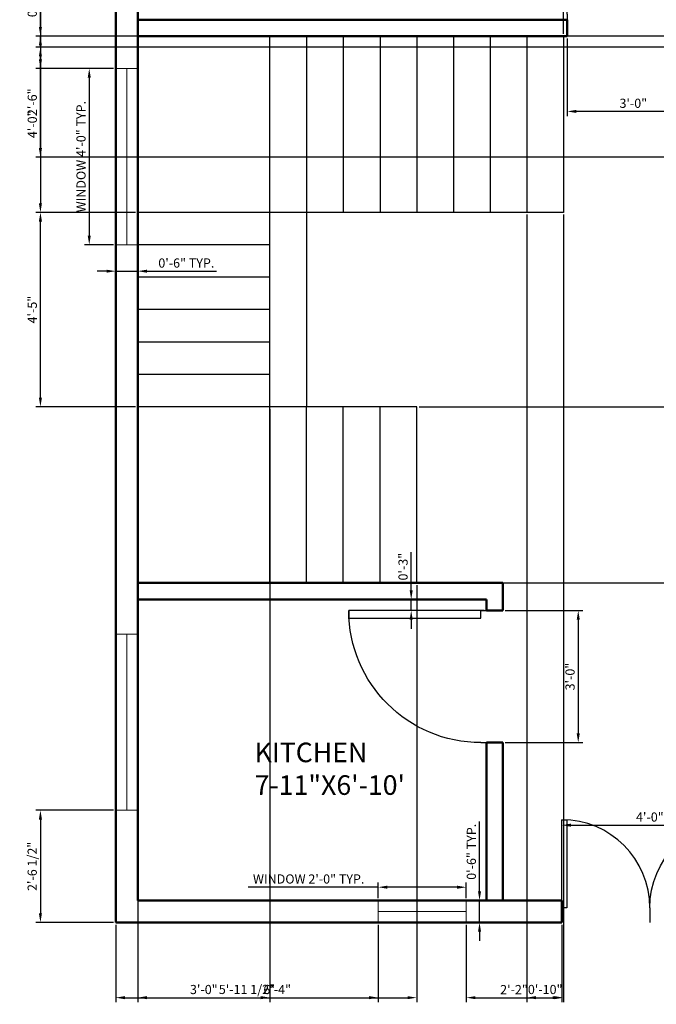
# Model space of a CAD drawing. Units: inches. Extents: x 158445 to 158806, y 254100 to 254533.
# Tile 1 of 3: x 158445 to 158619, y 254100 to 254369. Entities that reach past the tile are written whole.
import ezdxf

# ---------------------------------------------------------------- set-up
doc = ezdxf.new("R2010")
doc.units = ezdxf.units.IN
for name, color, linetype, lineweight in [('A-ANNO-DIMS', 2, 'Continuous', 18), ('A-AREA-IDEN', 7, 'Continuous', 25), ('A-DOOR', 3, 'Continuous', 25), ('A-FLOR-STRS', 7, 'Continuous', 25), ('A-GLAZ', 4, 'Continuous', 18), ('A-WALL', 7, 'Continuous', 50)]:
    doc.layers.add(name, color=color, linetype=linetype, lineweight=lineweight)
doc.styles.get("Standard").update_dxf_attribs({"font": 'arial.ttf'})
doc.dimstyles.new('ISO-25', dxfattribs={"dimtxt": 2.5, "dimasz": 2.5, "dimexe": 1.25, "dimexo": 0.625, "dimtad": 1, "dimlunit": 4, "dimtxsty": 'Standard', "dimcen": 2.5, "dimadec": 0, "dimazin": 0, "dimtfac": 1, "dimtmove": 0, "dimatfit": 3, "dimfxl": 1, "dimarcsym": 0})

# ---------------------------------------------------------------- blocks, each defined once
blk = doc.blocks.new('*U2')
for p, q in [((0, 0), (0, -5)), ((30, 0), (30, -5))]:
    blk.add_line(p, q)
blk.add_lwpolyline([(0, 0), (0, 30), (1.75, 30), (1.75, 0)], close=True)
blk.add_arc((0, 0), 30, 0, 90)
blk = doc.blocks.new('WIN-48IN')
for p, q in [((0, 6), (0, 0)), ((48, 6), (48, 0)), ((0, 3), (48, 3))]:
    blk.add_line(p, q)
blk = doc.blocks.new('WIN-24IN')
for p, q in [((0, 24), (6, 24)), ((3, 0), (3, 24)), ((0, 0), (6, 0))]:
    blk.add_line(p, q)
blk = doc.blocks.new('*D12')
at = {"layer": 'A-ANNO-DIMS', "color": 0, "lineweight": -2, "transparency": 16777216}
for p, q in [((158470.76, 254355.39), (158462.93, 254355.39)), ((158464.18, 254352.89), (158464.18, 254309.89)), ((158470.76, 254307.39), (158462.93, 254307.39))]:
    blk.add_line(p, q, dxfattribs=at)
at = {"layer": 'A-ANNO-DIMS', "color": 0, "transparency": 16777216}
for points in [[(158463.76, 254352.89), (158464.6, 254352.89), (158464.18, 254355.39)], [(158463.76, 254309.89), (158464.6, 254309.89), (158464.18, 254307.39)]]:
    blk.add_solid(points, dxfattribs=at)
at = {"layer": 'Defpoints', "color": 0, "transparency": 16777216}
for p in [(158471.38, 254355.39), (158464.18, 254307.39), (158471.38, 254307.39)]:
    blk.add_point(p, dxfattribs=at)
at = {"layer": 'A-ANNO-DIMS', "color": 0, "transparency": 16777216, "insert": (158462.26, 254331.39), "char_height": 2.5, "attachment_point": 5, "rotation": 90}
blk.add_mtext('WINDOW 4\'-0" TYP.', dxfattribs=at)
blk = doc.blocks.new('*D13')
at = {"layer": 'A-ANNO-DIMS', "color": 0, "lineweight": -2, "transparency": 16777216}
for p, q in [((158471.38, 254306.76), (158471.38, 254298.94)), ((158477.38, 254306.76), (158477.38, 254298.94)), ((158468.88, 254300.19), (158466.38, 254300.19)), ((158471.38, 254300.19), (158477.38, 254300.19)), ((158479.88, 254300.19), (158498.87, 254300.19))]:
    blk.add_line(p, q, dxfattribs=at)
at = {"layer": 'A-ANNO-DIMS', "color": 0, "transparency": 16777216}
for points in [[(158468.88, 254300.6), (158468.88, 254299.77), (158471.38, 254300.19)], [(158479.88, 254300.6), (158479.88, 254299.77), (158477.38, 254300.19)]]:
    blk.add_solid(points, dxfattribs=at)
at = {"layer": 'Defpoints', "color": 0, "transparency": 16777216}
for p in [(158471.38, 254307.39), (158477.38, 254307.39), (158477.38, 254300.19)]:
    blk.add_point(p, dxfattribs=at)
at = {"layer": 'A-ANNO-DIMS', "color": 0, "transparency": 16777216, "insert": (158490.63, 254302.09), "char_height": 2.5, "attachment_point": 5}
blk.add_mtext('0\'-6" TYP.', dxfattribs=at)
blk = doc.blocks.new('*D14')
at = {"layer": 'A-ANNO-DIMS', "color": 0, "lineweight": -2, "transparency": 16777216}
for p, q in [((158542.89, 254129.35), (158542.89, 254133.57)), ((158566.89, 254129.35), (158566.89, 254133.57)), ((158542.89, 254132.32), (158507.5, 254132.32)), ((158564.39, 254132.32), (158545.39, 254132.32))]:
    blk.add_line(p, q, dxfattribs=at)
at = {"layer": 'A-ANNO-DIMS', "color": 0, "transparency": 16777216}
for points in [[(158545.39, 254132.74), (158545.39, 254131.9), (158542.89, 254132.32)], [(158564.39, 254132.74), (158564.39, 254131.9), (158566.89, 254132.32)]]:
    blk.add_solid(points, dxfattribs=at)
at = {"layer": 'Defpoints', "color": 0, "transparency": 16777216}
for p in [(158542.89, 254132.32), (158542.89, 254128.72), (158566.89, 254128.72)]:
    blk.add_point(p, dxfattribs=at)
at = {"layer": 'A-ANNO-DIMS', "color": 0, "transparency": 16777216, "insert": (158523.95, 254134.24), "char_height": 2.5, "attachment_point": 5}
blk.add_mtext('WINDOW 2\'-0" TYP.', dxfattribs=at)
blk = doc.blocks.new('*D15')
at = {"layer": 'A-ANNO-DIMS', "color": 0, "lineweight": -2, "transparency": 16777216}
for p, q in [((158570.49, 254131.22), (158570.49, 254150.21)), ((158567.51, 254128.72), (158571.74, 254128.72)), ((158570.49, 254122.72), (158570.49, 254128.72)), ((158567.51, 254122.72), (158571.74, 254122.72)), ((158570.49, 254120.22), (158570.49, 254117.72))]:
    blk.add_line(p, q, dxfattribs=at)
at = {"layer": 'A-ANNO-DIMS', "color": 0, "transparency": 16777216}
for points in [[(158570.07, 254131.22), (158570.91, 254131.22), (158570.49, 254128.72)], [(158570.07, 254120.22), (158570.91, 254120.22), (158570.49, 254122.72)]]:
    blk.add_solid(points, dxfattribs=at)
at = {"layer": 'Defpoints', "color": 0, "transparency": 16777216}
for p in [(158566.89, 254128.72), (158570.49, 254128.72), (158566.89, 254122.72)]:
    blk.add_point(p, dxfattribs=at)
at = {"layer": 'A-ANNO-DIMS', "color": 0, "transparency": 16777216, "insert": (158568.59, 254141.97), "char_height": 2.5, "attachment_point": 5, "rotation": 90}
blk.add_mtext('0\'-6" TYP.', dxfattribs=at)
blk = doc.blocks.new('*D19')
at = {"layer": 'A-ANNO-DIMS', "color": 0, "lineweight": -2, "transparency": 16777216}
for p, q in [((158470.76, 254399.48), (158449.63, 254399.48)), ((158450.88, 254396.98), (158450.88, 254357.89)), ((158470.76, 254355.39), (158449.63, 254355.39))]:
    blk.add_line(p, q, dxfattribs=at)
at = {"layer": 'A-ANNO-DIMS', "color": 0, "transparency": 16777216}
for points in [[(158450.46, 254396.98), (158451.3, 254396.98), (158450.88, 254399.48)], [(158450.46, 254357.89), (158451.3, 254357.89), (158450.88, 254355.39)]]:
    blk.add_solid(points, dxfattribs=at)
at = {"layer": 'Defpoints', "color": 0, "transparency": 16777216}
for p in [(158471.38, 254399.48), (158450.88, 254355.39), (158471.38, 254355.39)]:
    blk.add_point(p, dxfattribs=at)
at = {"layer": 'A-ANNO-DIMS', "color": 0, "transparency": 16777216, "insert": (158448.98, 254377.43), "char_height": 2.5, "attachment_point": 5, "rotation": 90}
blk.add_mtext('3\'-8"', dxfattribs=at)
blk = doc.blocks.new('*D20')
at = {"layer": 'A-ANNO-DIMS', "color": 0, "lineweight": -2, "transparency": 16777216}
for p, q in [((158470.76, 254153.27), (158449.63, 254153.27)), ((158450.88, 254150.77), (158450.88, 254125.22)), ((158470.76, 254122.72), (158449.63, 254122.72))]:
    blk.add_line(p, q, dxfattribs=at)
at = {"layer": 'A-ANNO-DIMS', "color": 0, "transparency": 16777216}
for points in [[(158450.46, 254150.77), (158451.3, 254150.77), (158450.88, 254153.27)], [(158450.46, 254125.22), (158451.3, 254125.22), (158450.88, 254122.72)]]:
    blk.add_solid(points, dxfattribs=at)
at = {"layer": 'Defpoints', "color": 0, "transparency": 16777216}
for p in [(158471.38, 254153.27), (158450.88, 254122.72), (158471.38, 254122.72)]:
    blk.add_point(p, dxfattribs=at)
at = {"layer": 'A-ANNO-DIMS', "color": 0, "transparency": 16777216, "insert": (158448.96, 254138), "char_height": 2.5, "attachment_point": 5, "rotation": 90}
blk.add_mtext('2\'-6 1/2"', dxfattribs=at)
blk = doc.blocks.new('*D23')
at = {"layer": 'A-ANNO-DIMS', "color": 0, "lineweight": -2, "transparency": 16777216}
for p, q in [((158471.38, 254122.1), (158471.38, 254100.97)), ((158542.89, 254122.1), (158542.89, 254100.97)), ((158473.88, 254102.22), (158540.39, 254102.22))]:
    blk.add_line(p, q, dxfattribs=at)
at = {"layer": 'A-ANNO-DIMS', "color": 0, "transparency": 16777216}
for points in [[(158473.88, 254102.64), (158473.88, 254101.8), (158471.38, 254102.22)], [(158540.39, 254102.64), (158540.39, 254101.8), (158542.89, 254102.22)]]:
    blk.add_solid(points, dxfattribs=at)
at = {"layer": 'Defpoints', "color": 0, "transparency": 16777216}
for p in [(158471.38, 254122.72), (158542.89, 254122.72), (158542.89, 254102.22)]:
    blk.add_point(p, dxfattribs=at)
at = {"layer": 'A-ANNO-DIMS', "color": 0, "transparency": 16777216, "insert": (158507.13, 254104.14), "char_height": 2.5, "attachment_point": 5}
blk.add_mtext('5\'-11 1/2"', dxfattribs=at)
blk = doc.blocks.new('*D24')
at = {"layer": 'A-ANNO-DIMS', "color": 0, "lineweight": -2, "transparency": 16777216}
for p, q in [((158566.89, 254122.1), (158566.89, 254100.97)), ((158592.88, 254122.1), (158592.88, 254100.97)), ((158569.39, 254102.22), (158590.38, 254102.22))]:
    blk.add_line(p, q, dxfattribs=at)
at = {"layer": 'A-ANNO-DIMS', "color": 0, "transparency": 16777216}
for points in [[(158569.39, 254102.64), (158569.39, 254101.8), (158566.89, 254102.22)], [(158590.38, 254102.64), (158590.38, 254101.8), (158592.88, 254102.22)]]:
    blk.add_solid(points, dxfattribs=at)
at = {"layer": 'Defpoints', "color": 0, "transparency": 16777216}
for p in [(158566.89, 254122.72), (158592.88, 254122.72), (158592.88, 254102.22)]:
    blk.add_point(p, dxfattribs=at)
at = {"layer": 'A-ANNO-DIMS', "color": 0, "transparency": 16777216, "insert": (158579.88, 254104.1), "char_height": 2.5, "attachment_point": 5}
blk.add_mtext('2\'-2"', dxfattribs=at)
blk = doc.blocks.new('*D25')
at = {"layer": 'A-ANNO-DIMS', "color": 0, "lineweight": -2, "transparency": 16777216}
for p, q in [((158592.88, 254129.35), (158592.88, 254150.47)), ((158595.38, 254149.22), (158638.38, 254149.22)), ((158640.88, 254129.35), (158640.88, 254150.47))]:
    blk.add_line(p, q, dxfattribs=at)
at = {"layer": 'A-ANNO-DIMS', "color": 0, "transparency": 16777216}
for points in [[(158595.38, 254149.64), (158595.38, 254148.8), (158592.88, 254149.22)], [(158638.38, 254149.64), (158638.38, 254148.8), (158640.88, 254149.22)]]:
    blk.add_solid(points, dxfattribs=at)
at = {"layer": 'Defpoints', "color": 0, "transparency": 16777216}
for p in [(158640.88, 254149.22), (158592.88, 254128.72), (158640.88, 254128.72)]:
    blk.add_point(p, dxfattribs=at)
at = {"layer": 'A-ANNO-DIMS', "color": 0, "transparency": 16777216, "insert": (158616.88, 254151.12), "char_height": 2.5, "attachment_point": 5}
blk.add_mtext('4\'-0"', dxfattribs=at)
blk = doc.blocks.new('*D29')
at = {"layer": 'A-ANNO-DIMS', "color": 0, "lineweight": -2, "transparency": 16777216}
for p, q in [((158728.76, 254361.22), (158449.63, 254361.22)), ((158450.88, 254333.72), (158450.88, 254358.72)), ((158728.76, 254331.22), (158449.63, 254331.22))]:
    blk.add_line(p, q, dxfattribs=at)
at = {"layer": 'A-ANNO-DIMS', "color": 0, "transparency": 16777216}
for points in [[(158450.46, 254358.72), (158451.3, 254358.72), (158450.88, 254361.22)], [(158450.46, 254333.72), (158451.3, 254333.72), (158450.88, 254331.22)]]:
    blk.add_solid(points, dxfattribs=at)
at = {"layer": 'Defpoints', "color": 0, "transparency": 16777216}
for p in [(158450.88, 254361.22), (158729.38, 254361.22), (158729.38, 254331.22)]:
    blk.add_point(p, dxfattribs=at)
at = {"layer": 'A-ANNO-DIMS', "color": 0, "transparency": 16777216, "insert": (158448.98, 254346.22), "char_height": 2.5, "attachment_point": 5, "rotation": 90}
blk.add_mtext('2\'-6"', dxfattribs=at)
blk = doc.blocks.new('*D30')
at = {"layer": 'A-ANNO-DIMS', "color": 0, "lineweight": -2, "transparency": 16777216}
for p, q in [((158477.38, 254364.85), (158477.38, 254528.47)), ((158593.38, 254364.85), (158593.38, 254528.47)), ((158479.88, 254527.22), (158590.88, 254527.22))]:
    blk.add_line(p, q, dxfattribs=at)
at = {"layer": 'A-ANNO-DIMS', "color": 0, "transparency": 16777216}
for points in [[(158479.88, 254527.64), (158479.88, 254526.8), (158477.38, 254527.22)], [(158590.88, 254527.64), (158590.88, 254526.8), (158593.38, 254527.22)]]:
    blk.add_solid(points, dxfattribs=at)
at = {"layer": 'Defpoints', "color": 0, "transparency": 16777216}
for p in [(158593.38, 254527.22), (158477.38, 254364.22), (158593.38, 254364.22)]:
    blk.add_point(p, dxfattribs=at)
at = {"layer": 'A-ANNO-DIMS', "color": 0, "transparency": 16777216, "insert": (158535.38, 254529.12), "char_height": 2.5, "attachment_point": 5}
blk.add_mtext('9\'-8"', dxfattribs=at)
blk = doc.blocks.new('*D31')
at = {"layer": 'A-ANNO-DIMS', "color": 0, "lineweight": -2, "transparency": 16777216}
for p, q in [((158476.76, 254364.22), (158449.63, 254364.22)), ((158450.88, 254361.72), (158450.88, 254318.72)), ((158476.76, 254316.22), (158449.63, 254316.22))]:
    blk.add_line(p, q, dxfattribs=at)
at = {"layer": 'A-ANNO-DIMS', "color": 0, "transparency": 16777216}
for points in [[(158450.46, 254361.72), (158451.3, 254361.72), (158450.88, 254364.22)], [(158450.46, 254318.72), (158451.3, 254318.72), (158450.88, 254316.22)]]:
    blk.add_solid(points, dxfattribs=at)
at = {"layer": 'Defpoints', "color": 0, "transparency": 16777216}
for p in [(158477.38, 254364.22), (158450.88, 254316.22), (158477.38, 254316.22)]:
    blk.add_point(p, dxfattribs=at)
at = {"layer": 'A-ANNO-DIMS', "color": 0, "transparency": 16777216, "insert": (158448.98, 254340.22), "char_height": 2.5, "attachment_point": 5, "rotation": 90}
blk.add_mtext('4\'-0"', dxfattribs=at)
blk = doc.blocks.new('*D32')
at = {"layer": 'A-ANNO-DIMS', "color": 0, "lineweight": -2, "transparency": 16777216}
for p, q in [((158477.38, 254214.6), (158477.38, 254100.97)), ((158553.38, 254214.6), (158553.38, 254100.97)), ((158479.88, 254102.22), (158550.88, 254102.22))]:
    blk.add_line(p, q, dxfattribs=at)
at = {"layer": 'A-ANNO-DIMS', "color": 0, "transparency": 16777216}
for points in [[(158479.88, 254102.64), (158479.88, 254101.8), (158477.38, 254102.22)], [(158550.88, 254102.64), (158550.88, 254101.8), (158553.38, 254102.22)]]:
    blk.add_solid(points, dxfattribs=at)
at = {"layer": 'Defpoints', "color": 0, "transparency": 16777216}
for p in [(158477.38, 254215.22), (158553.38, 254215.22), (158553.38, 254102.22)]:
    blk.add_point(p, dxfattribs=at)
at = {"layer": 'A-ANNO-DIMS', "color": 0, "transparency": 16777216, "insert": (158515.38, 254104.12), "char_height": 2.5, "attachment_point": 5}
blk.add_mtext('6\'-4"', dxfattribs=at)
blk = doc.blocks.new('*D33')
at = {"layer": 'A-ANNO-DIMS', "color": 0, "lineweight": -2, "transparency": 16777216}
for p, q in [((158477.38, 254262.6), (158477.38, 254100.97)), ((158513.38, 254262.6), (158513.38, 254100.97)), ((158479.88, 254102.22), (158510.88, 254102.22))]:
    blk.add_line(p, q, dxfattribs=at)
at = {"layer": 'A-ANNO-DIMS', "color": 0, "transparency": 16777216}
for points in [[(158479.88, 254102.64), (158479.88, 254101.8), (158477.38, 254102.22)], [(158510.88, 254102.64), (158510.88, 254101.8), (158513.38, 254102.22)]]:
    blk.add_solid(points, dxfattribs=at)
at = {"layer": 'Defpoints', "color": 0, "transparency": 16777216}
for p in [(158477.38, 254263.22), (158513.38, 254263.22), (158513.38, 254102.22)]:
    blk.add_point(p, dxfattribs=at)
at = {"layer": 'A-ANNO-DIMS', "color": 0, "transparency": 16777216, "insert": (158495.38, 254104.12), "char_height": 2.5, "attachment_point": 5}
blk.add_mtext('3\'-0"', dxfattribs=at)
blk = doc.blocks.new('*D34')
at = {"layer": 'A-ANNO-DIMS', "color": 0, "lineweight": -2, "transparency": 16777216}
for p, q in [((158554.01, 254263.22), (158805.13, 254263.22)), ((158803.88, 254260.72), (158803.88, 254217.72)), ((158554.01, 254215.22), (158805.13, 254215.22))]:
    blk.add_line(p, q, dxfattribs=at)
at = {"layer": 'A-ANNO-DIMS', "color": 0, "transparency": 16777216}
for points in [[(158803.46, 254260.72), (158804.3, 254260.72), (158803.88, 254263.22)], [(158803.46, 254217.72), (158804.3, 254217.72), (158803.88, 254215.22)]]:
    blk.add_solid(points, dxfattribs=at)
at = {"layer": 'Defpoints', "color": 0, "transparency": 16777216}
for p in [(158553.38, 254263.22), (158553.38, 254215.22), (158803.88, 254215.22)]:
    blk.add_point(p, dxfattribs=at)
at = {"layer": 'A-ANNO-DIMS', "color": 0, "transparency": 16777216, "insert": (158801.98, 254239.22), "char_height": 2.5, "attachment_point": 5, "rotation": 90}
blk.add_mtext('4\'-0"', dxfattribs=at)
blk = doc.blocks.new('*D35')
at = {"layer": 'A-ANNO-DIMS', "color": 0, "lineweight": -2, "transparency": 16777216}
for p, q in [((158583.38, 254315.6), (158583.38, 254100.97)), ((158593.38, 254315.6), (158593.38, 254100.97)), ((158585.88, 254102.22), (158590.88, 254102.22))]:
    blk.add_line(p, q, dxfattribs=at)
at = {"layer": 'A-ANNO-DIMS', "color": 0, "transparency": 16777216}
for points in [[(158585.88, 254102.64), (158585.88, 254101.8), (158583.38, 254102.22)], [(158590.88, 254102.64), (158590.88, 254101.8), (158593.38, 254102.22)]]:
    blk.add_solid(points, dxfattribs=at)
at = {"layer": 'Defpoints', "color": 0, "transparency": 16777216}
for p in [(158583.38, 254316.22), (158593.38, 254316.22), (158593.38, 254102.22)]:
    blk.add_point(p, dxfattribs=at)
at = {"layer": 'A-ANNO-DIMS', "color": 0, "transparency": 16777216, "insert": (158588.38, 254104.12), "char_height": 2.5, "attachment_point": 5}
blk.add_mtext('0\'-10"', dxfattribs=at)
blk = doc.blocks.new('*D36')
at = {"layer": 'A-ANNO-DIMS', "color": 0, "lineweight": -2, "transparency": 16777216}
for p, q in [((158476.76, 254316.22), (158449.63, 254316.22)), ((158450.88, 254265.72), (158450.88, 254313.72)), ((158476.76, 254263.22), (158449.63, 254263.22))]:
    blk.add_line(p, q, dxfattribs=at)
at = {"layer": 'A-ANNO-DIMS', "color": 0, "transparency": 16777216}
for points in [[(158450.46, 254313.72), (158451.3, 254313.72), (158450.88, 254316.22)], [(158450.46, 254265.72), (158451.3, 254265.72), (158450.88, 254263.22)]]:
    blk.add_solid(points, dxfattribs=at)
at = {"layer": 'Defpoints', "color": 0, "transparency": 16777216}
for p in [(158450.88, 254316.22), (158477.38, 254316.22), (158477.38, 254263.22)]:
    blk.add_point(p, dxfattribs=at)
at = {"layer": 'A-ANNO-DIMS', "color": 0, "transparency": 16777216, "insert": (158448.98, 254289.72), "char_height": 2.5, "attachment_point": 5, "rotation": 90}
blk.add_mtext('4\'-5"', dxfattribs=at)
blk = doc.blocks.new('*D40')
at = {"layer": 'A-ANNO-DIMS', "color": 0, "lineweight": -2, "transparency": 16777216}
for p, q in [((158594.38, 254363.6), (158594.38, 254342.47)), ((158630.38, 254363.6), (158630.38, 254342.47)), ((158627.88, 254343.72), (158596.88, 254343.72))]:
    blk.add_line(p, q, dxfattribs=at)
at = {"layer": 'A-ANNO-DIMS', "color": 0, "transparency": 16777216}
for points in [[(158596.88, 254344.14), (158596.88, 254343.3), (158594.38, 254343.72)], [(158627.88, 254344.14), (158627.88, 254343.3), (158630.38, 254343.72)]]:
    blk.add_solid(points, dxfattribs=at)
at = {"layer": 'Defpoints', "color": 0, "transparency": 16777216}
for p in [(158594.38, 254364.22), (158630.38, 254364.22), (158594.38, 254343.72)]:
    blk.add_point(p, dxfattribs=at)
at = {"layer": 'A-ANNO-DIMS', "color": 0, "transparency": 16777216, "insert": (158612.38, 254345.62), "char_height": 2.5, "attachment_point": 5}
blk.add_mtext('3\'-0"', dxfattribs=at)
blk = doc.blocks.new('*D42')
at = {"layer": 'A-ANNO-DIMS', "color": 0, "lineweight": -2, "transparency": 16777216}
for p, q in [((158577.51, 254207.72), (158598.63, 254207.72)), ((158597.38, 254205.22), (158597.38, 254174.22)), ((158577.51, 254171.72), (158598.63, 254171.72))]:
    blk.add_line(p, q, dxfattribs=at)
at = {"layer": 'A-ANNO-DIMS', "color": 0, "transparency": 16777216}
for points in [[(158596.96, 254205.22), (158597.8, 254205.22), (158597.38, 254207.72)], [(158596.96, 254174.22), (158597.8, 254174.22), (158597.38, 254171.72)]]:
    blk.add_solid(points, dxfattribs=at)
at = {"layer": 'Defpoints', "color": 0, "transparency": 16777216}
for p in [(158576.88, 254207.72), (158576.88, 254171.72), (158597.38, 254171.72)]:
    blk.add_point(p, dxfattribs=at)
at = {"layer": 'A-ANNO-DIMS', "color": 0, "transparency": 16777216, "insert": (158595.48, 254189.72), "char_height": 2.5, "attachment_point": 5, "rotation": 90}
blk.add_mtext('3\'-0"', dxfattribs=at)
blk = doc.blocks.new('*D51')
at = {"layer": 'A-ANNO-DIMS', "color": 0, "lineweight": -2, "transparency": 16777216}
for p, q in [((158551.88, 254213.22), (158551.88, 254223.62)), ((158571.76, 254210.72), (158550.63, 254210.72)), ((158551.88, 254207.72), (158551.88, 254210.72)), ((158571.76, 254207.72), (158550.63, 254207.72)), ((158551.88, 254205.22), (158551.88, 254202.72))]:
    blk.add_line(p, q, dxfattribs=at)
at = {"layer": 'A-ANNO-DIMS', "color": 0, "transparency": 16777216}
for points in [[(158551.46, 254213.22), (158552.3, 254213.22), (158551.88, 254210.72)], [(158551.46, 254205.22), (158552.3, 254205.22), (158551.88, 254207.72)]]:
    blk.add_solid(points, dxfattribs=at)
at = {"layer": 'Defpoints', "color": 0, "transparency": 16777216}
for p in [(158551.88, 254210.72), (158572.38, 254210.72), (158572.38, 254207.72)]:
    blk.add_point(p, dxfattribs=at)
at = {"layer": 'A-ANNO-DIMS', "color": 0, "transparency": 16777216, "insert": (158549.98, 254219.67), "char_height": 2.5, "attachment_point": 5, "rotation": 90}
blk.add_mtext('0\'-3"', dxfattribs=at)
blk = doc.blocks.new('*D53')
at = {"layer": 'A-ANNO-DIMS', "color": 0, "lineweight": -2, "transparency": 16777216}
for p, q in [((158450.88, 254366.72), (158450.88, 254377.12)), ((158728.76, 254364.22), (158449.63, 254364.22)), ((158450.88, 254361.22), (158450.88, 254364.22)), ((158728.76, 254361.22), (158449.63, 254361.22)), ((158450.88, 254358.72), (158450.88, 254356.22))]:
    blk.add_line(p, q, dxfattribs=at)
at = {"layer": 'A-ANNO-DIMS', "color": 0, "transparency": 16777216}
for points in [[(158450.46, 254366.72), (158451.3, 254366.72), (158450.88, 254364.22)], [(158450.46, 254358.72), (158451.3, 254358.72), (158450.88, 254361.22)]]:
    blk.add_solid(points, dxfattribs=at)
at = {"layer": 'Defpoints', "color": 0, "transparency": 16777216}
for p in [(158450.88, 254364.22), (158729.38, 254364.22), (158729.38, 254361.22)]:
    blk.add_point(p, dxfattribs=at)
at = {"layer": 'A-ANNO-DIMS', "color": 0, "transparency": 16777216, "insert": (158448.98, 254373.17), "char_height": 2.5, "attachment_point": 5, "rotation": 90}
blk.add_mtext('0\'-3"', dxfattribs=at)

msp = doc.modelspace()

# ---------------------------------------------------------------- linework, layer by layer
at = {"layer": 'A-FLOR-STRS'}
for p, q in [((158513.381, 254215.221), (158513.381, 254364.221)), ((158523.381, 254364.221), (158523.381, 254263.221)), ((158523.381, 254364.221), (158523.381, 254316.221)), ((158533.381, 254364.221), (158533.381, 254316.221)), ((158543.381, 254364.221), (158543.381, 254316.221)), ((158553.381, 254364.221), (158553.381, 254316.221)), ((158563.381, 254364.221), (158563.381, 254316.221)), ((158573.381, 254364.221), (158573.381, 254316.221)), ((158583.381, 254364.221), (158583.381, 254316.221)), ((158593.381, 254364.221), (158593.381, 254316.221)), ((158523.381, 254316.221), (158477.381, 254316.221)), ((158593.381, 254316.221), (158523.381, 254316.221)), ((158513.381, 254307.388), (158477.381, 254307.388)), ((158513.381, 254298.554), (158477.381, 254298.554)), ((158513.381, 254289.721), (158477.381, 254289.721)), ((158513.381, 254280.888), (158477.381, 254280.888)), ((158513.381, 254272.054), (158477.381, 254272.054)), ((158513.381, 254263.221), (158477.381, 254263.221)), ((158523.381, 254263.221), (158477.381, 254263.221)), ((158553.381, 254263.221), (158523.381, 254263.221)), ((158523.381, 254215.221), (158523.381, 254263.221)), ((158533.381, 254215.221), (158533.381, 254263.221)), ((158543.381, 254215.221), (158543.381, 254263.221)), ((158553.381, 254215.221), (158553.381, 254263.221))]:
    msp.add_line(p, q, dxfattribs=at)
at = {"layer": 'A-WALL'}
for p, q in [((158471.381, 254506.721), (158471.381, 254122.721)), ((158477.381, 254500.721), (158477.381, 254368.721)), ((158477.381, 254368.721), (158477.381, 254268.721)), ((158594.381, 254368.721), (158477.381, 254368.721)), ((158594.381, 254364.221), (158594.381, 254368.721)), ((158594.381, 254364.221), (158477.381, 254364.221)), ((158477.381, 254268.721), (158477.381, 254128.721)), ((158477.381, 254215.221), (158576.881, 254215.221)), ((158576.881, 254215.221), (158576.881, 254207.721)), ((158477.381, 254210.721), (158572.381, 254210.721)), ((158572.381, 254210.721), (158572.381, 254207.721)), ((158572.381, 254210.721), (158572.381, 254207.721)), ((158572.381, 254207.721), (158576.881, 254207.721)), ((158576.881, 254171.721), (158572.381, 254171.721)), ((158572.381, 254171.721), (158572.381, 254128.721)), ((158576.881, 254171.721), (158576.881, 254128.721)), ((158477.381, 254128.721), (158592.881, 254128.721)), ((158592.881, 254122.721), (158592.881, 254128.721)), ((158471.381, 254122.721), (158592.881, 254122.721))]:
    msp.add_line(p, q, dxfattribs=at)

# ---------------------------------------------------------------- block references
at = {"layer": 'A-DOOR'}
for p, xscale, yscale, zscale in [((158630.381, 254370.221), -1.199999999999999, 1.199999999999999, 1.199999999999999), ((158592.881, 254126.721), 0.8, 0.8, 0.8), ((158640.881, 254126.721), -0.8, 0.8, 0.8)]:
    msp.add_blockref('*U2', p, dxfattribs=dict(at, xscale=xscale, yscale=yscale, zscale=zscale))
at = {"layer": 'A-DOOR', "xscale": -1.199999999999999, "yscale": 1.199999999999999, "zscale": 1.199999999999999, "rotation": 90}
msp.add_blockref('*U2', (158570.881, 254207.721), dxfattribs=at)
at = {"layer": 'A-GLAZ'}
for name, p, rotation in [('WIN-48IN', (158471.381, 254355.388), 269.9999999998033), ('WIN-48IN', (158471.381, 254201.27), 269.9999999998119), ('WIN-24IN', (158566.889, 254122.721), 89.9999999998038)]:
    msp.add_blockref(name, p, dxfattribs=dict(at, rotation=rotation))

# ---------------------------------------------------------------- texts
at = {"layer": 'A-AREA-IDEN', "insert": (158509.227, 254171.717), "char_height": 5.335, "attachment_point": 1}
msp.add_mtext_dynamic_manual_height_columns('KITCHEN\\P7-11"X6\'-10\'', width=5.37287, gutter_width=26.675, heights=[0], dxfattribs=at)

# ---------------------------------------------------------------- dimensions: what is measured, and where the dimension line sits
at = {"layer": 'A-ANNO-DIMS'}
for base, p1, p2, picture, middle in [((158593.381, 254527.221), (158477.381, 254364.221), (158593.381, 254364.221), '*D30', (158535.381, 254529.122)), ((158593.381, 254102.221), (158583.381, 254316.221), (158593.381, 254316.221), '*D35', (158588.381, 254104.122)), ((158513.381, 254102.221), (158477.381, 254263.221), (158513.381, 254263.221), '*D33', (158495.381, 254104.123)), ((158553.381, 254102.221), (158477.381, 254215.221), (158553.381, 254215.221), '*D32', (158515.381, 254104.122)), ((158640.881, 254149.221), (158592.881, 254128.721), (158640.881, 254128.721), '*D25', (158616.881, 254151.122)), ((158542.889, 254102.221), (158471.381, 254122.721), (158542.889, 254122.721), '*D23', (158507.135, 254104.139)), ((158592.881, 254102.221), (158566.889, 254122.721), (158592.881, 254122.721), '*D24', (158579.885, 254104.101))]:
    dim = msp.add_linear_dim(base=base, p1=p1, p2=p2, dimstyle='ISO-25', override={"dimdec": 1, "dimlfac": 1, "dimrnd": 0, "dimzin": 1, "dimdsep": 46, "dimlunit": 4, "dimfrac": 2}, dxfattribs=at)
    dim.commit()
    dim.dimension.update_dxf_attribs({"geometry": picture, "text_midpoint": middle})
for base, p1, p2, angle, picture, middle in [((158450.881, 254355.388), (158471.381, 254399.482), (158471.381, 254355.388), 90, '*D19', (158448.979, 254377.435)), ((158450.881, 254364.221), (158729.381, 254361.221), (158729.381, 254364.221), 90, '*D53', (158448.979, 254373.169)), ((158450.881, 254316.221), (158477.381, 254364.221), (158477.381, 254316.221), 90, '*D31', (158448.98, 254340.221)), ((158594.381, 254343.721), (158630.381, 254364.221), (158594.381, 254364.221), 180, '*D40', (158612.381, 254345.623)), ((158450.881, 254361.221), (158729.381, 254331.221), (158729.381, 254361.221), 90, '*D29', (158448.98, 254346.221)), ((158450.881, 254316.221), (158477.381, 254263.221), (158477.381, 254316.221), 90, '*D36', (158448.985, 254289.721)), ((158803.881, 254215.221), (158553.381, 254263.221), (158553.381, 254215.221), 90, '*D34', (158801.98, 254239.221)), ((158551.881, 254210.721), (158572.381, 254207.721), (158572.381, 254210.721), 90, '*D51', (158549.979, 254219.669)), ((158597.381, 254171.721), (158576.881, 254207.721), (158576.881, 254171.721), 270, '*D42', (158595.479, 254189.721)), ((158450.881, 254122.721), (158471.381, 254153.27), (158471.381, 254122.721), 90, '*D20', (158448.964, 254137.995))]:
    dim = msp.add_linear_dim(base=base, p1=p1, p2=p2, angle=angle, dimstyle='ISO-25', override={"dimdec": 1, "dimlfac": 1, "dimrnd": 0, "dimzin": 1, "dimdsep": 46, "dimlunit": 4, "dimfrac": 2}, dxfattribs=at)
    dim.commit()
    dim.dimension.update_dxf_attribs({"geometry": picture, "text_midpoint": middle})
for base, p1, p2, angle, text, picture, middle in [((158464.181, 254307.388), (158471.381, 254355.388), (158471.381, 254307.388), 270, 'WINDOW <> TYP.', '*D12', (158462.263, 254331.388)), ((158570.489, 254128.721), (158566.889, 254122.721), (158566.889, 254128.721), 90, '<> TYP.', '*D15', (158568.587, 254141.965)), ((158542.889, 254132.321), (158566.889, 254128.721), (158542.889, 254128.721), 180, 'WINDOW <> TYP.', '*D14', (158523.946, 254134.239))]:
    dim = msp.add_linear_dim(base=base, p1=p1, p2=p2, angle=angle, text=text, dimstyle='ISO-25', override={"dimdec": 1, "dimlfac": 1, "dimrnd": 0, "dimzin": 1, "dimdsep": 46, "dimlunit": 4, "dimfrac": 2}, dxfattribs=at)
    dim.commit()
    dim.dimension.update_dxf_attribs({"geometry": picture, "text_midpoint": middle})
dim = msp.add_linear_dim(base=(158477.381, 254300.188), p1=(158471.381, 254307.388), p2=(158477.381, 254307.388), text='<> TYP.', dimstyle='ISO-25', override={"dimdec": 1, "dimlfac": 1, "dimrnd": 0, "dimzin": 1, "dimdsep": 46, "dimlunit": 4, "dimfrac": 2}, dxfattribs=at)
dim.commit()
dim.dimension.update_dxf_attribs({"geometry": '*D13', "text_midpoint": (158490.626, 254302.089)})

doc.saveas('drawing.dxf')
